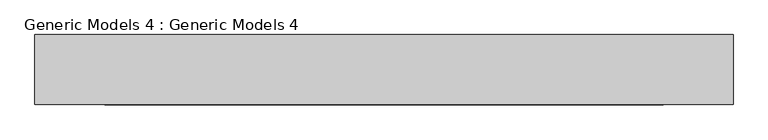
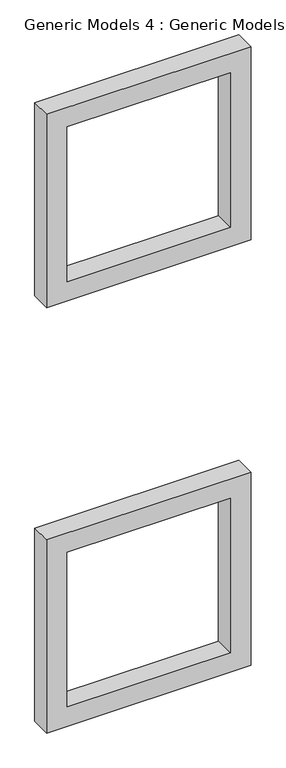
"""IFC4 building model written with IfcOpenShell, lengths in millimetres: proxy geometry, Generic Models 4 : Generic Models 4."""

from ifc_helpers import new_model, si_unit, frame, origin, place, context, project, spatial, polyline, outline, extrude, source, transform, mapped, element, save


def generic_models_4_generic_models_4_fb6d851a(model_context):
    return source(origin(), model_context, "Body", "SweptSolid", [
        extrude(outline(polyline([(5943.6, -12309.6023867), (4419.6, -12309.6023867), (4419.6, -10785.6023867), (5943.6, -10785.6023867), (5943.6, -12309.6023867)]), holes=[polyline([(5791.2, -10938.0023867), (4572.0, -10938.0023867), (4572.0, -12157.2023867), (5791.2, -12157.2023867), (5791.2, -10938.0023867)])]), frame((0.0, -673.9499863, 0.0), z_axis=(0.0, 1.0, 0.0), x_axis=(0.0, 0.0, 1.0)), (0.0, 0.0, 1.0), 152.4),
        extrude(outline(polyline([(1066.8, -10785.6023867), (2590.8, -10785.6023867), (2590.8, -12309.6023867), (1066.8, -12309.6023867), (1066.8, -10785.6023867)]), holes=[polyline([(2438.4, -10938.0023867), (1219.2, -10938.0023867), (1219.2, -12157.2023867), (2438.4, -12157.2023867), (2438.4, -10938.0023867)])]), frame((0.0, -673.9499863, 0.0), z_axis=(0.0, 1.0, 0.0), x_axis=(0.0, 0.0, 1.0)), (0.0, 0.0, 1.0), 152.4),
    ])


if __name__ == "__main__":
    model = new_model("IFC4")
    model_context = context("Model", 3, world=origin())
    ifc_project = project(units=[si_unit("LENGTHUNIT", "METRE", prefix="MILLI")], contexts=[model_context])
    site = spatial("IfcSite", under=ifc_project)
    building = spatial("IfcBuilding", under=site)
    placement = place(None, origin())
    generic_models_4_generic_models_4_shape = generic_models_4_generic_models_4_fb6d851a(model_context)
    element("IfcBuildingElementProxy", 1, Name="Generic Models 4 : Generic Models 4", ObjectType="Generic Models 4 : Generic Models 4", at=placement, inside=building, context=model_context, shape_type="MappedRepresentation", body=[
        mapped(generic_models_4_generic_models_4_shape, transform((0.0, 0.0, 0.0), x_axis=(1.0, 0.0, 0.0), y_axis=(0.0, 1.0, 0.0), z_axis=(0.0, 0.0, 1.0))),
    ])
    save(model, "model.ifc")

# Revit data of these elements
# Element 1 (IfcBuildingElementProxy, "Generic Models 4 : Generic Models 4")
#   Materials on its faces: "accent wall"
# Materials
#   "accent wall": class "Generic", colour RGB 120 120 120, transparency 0, Cost = 0
